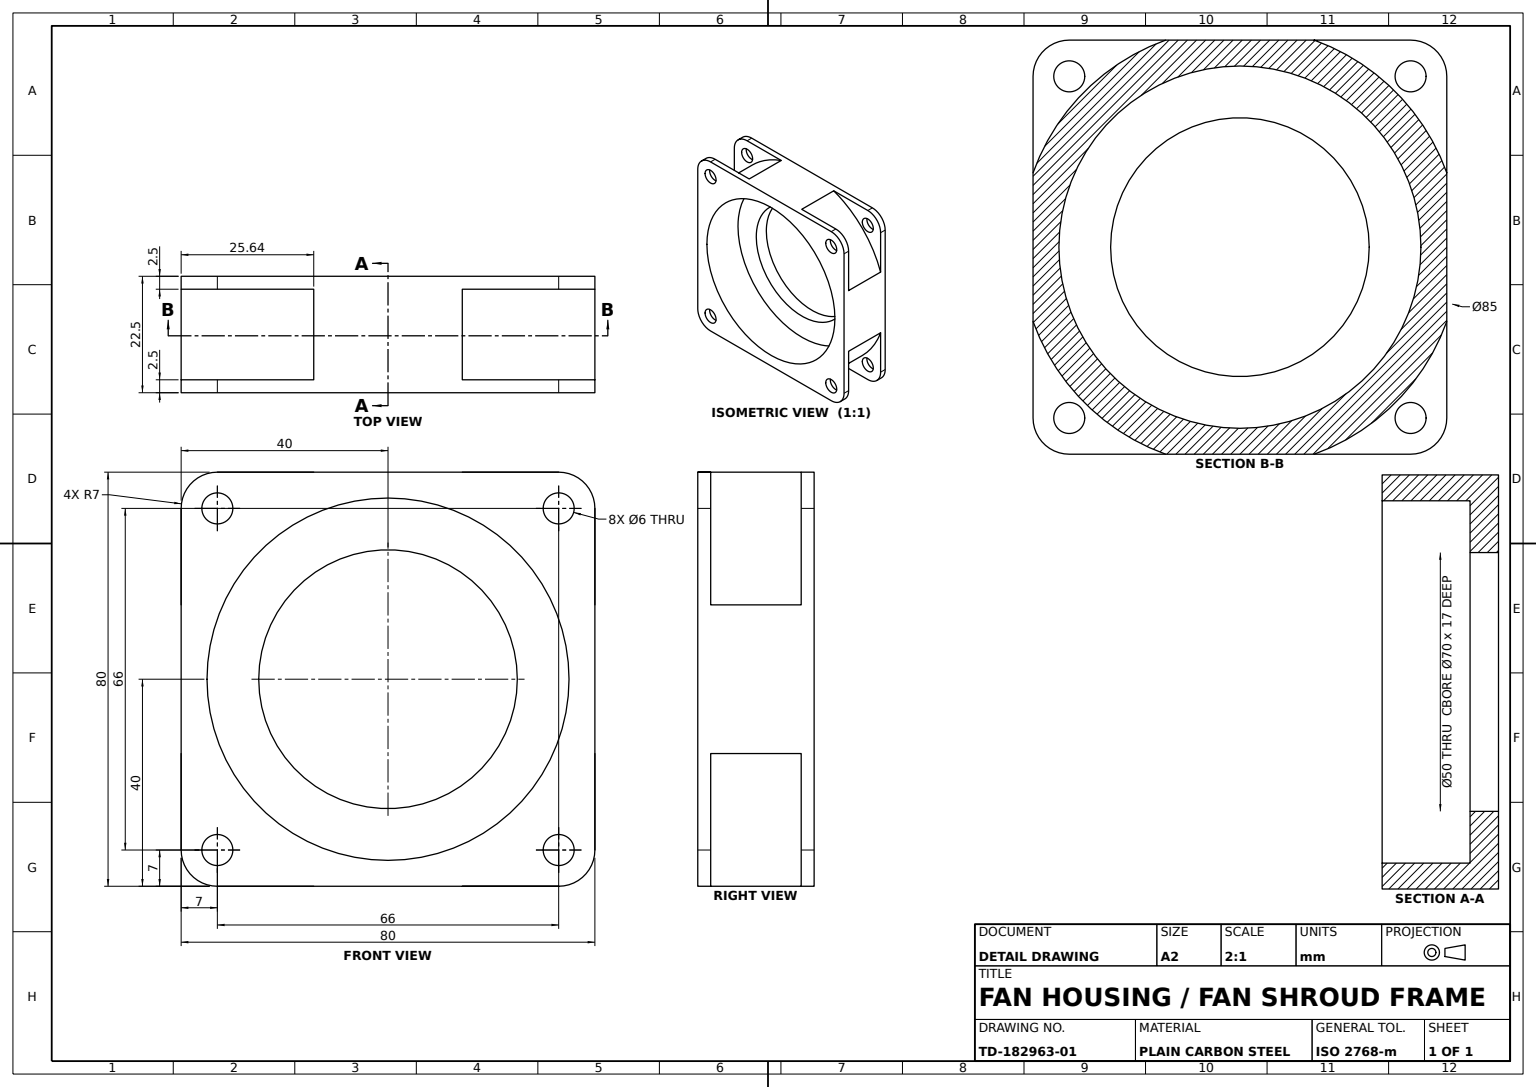
SolidWorks part; units mm, degrees
material "Plain Carbon Steel"
ref_plane "Front Plane" through (0, 0, 0) normal (0, 0, 1) x (1, 0, 0)
ref_plane "Top Plane" through (0, 0, 0) normal (0, 1, 0) x (1, 0, 0)
ref_plane "Right Plane" through (0, 0, 0) normal (1, 0, 0) x (0, 0, -1)
sketch "Front Flange Sketch" plane through (0, 0, 0) normal (0, 0, 1) x (1, 0, 0)
  line L0 (0, 0) -> (33, 0)
  line L1 (40, 7) -> (40, 73)
  line L2 (33, 80) -> (-33, 80)
  line L3 (-40, 73) -> (-40, 7)
  line L4 (-33, 0) -> (0, 0)
  arc A0 (33, 0) -> (40, 7) centre (33, 7) ccw
  arc A1 (-33, 0) -> (-40, 7) centre (-33, 7) cw
  arc A2 (40, 73) -> (33, 80) centre (33, 73) ccw
  arc A3 (-40, 73) -> (-33, 80) centre (-33, 73) cw
  point P8 (40, 0)
  point P11 (-40, 0)
  point P14 (40, 80)
  point P17 (-40, 80)
  dimension "D5" = 7
  dimension "D1" = 40
  dimension "D2" = 80
  dimension "D3" = 80
  dimension "D4" = 80
extrude "Front Flange 80x80" add sketch "Front Flange Sketch" along normal blind 2.5
sketch "Hub Sketch" plane through (0, 0, 2.5) normal (0, 0, 1) x (1, 0, 0)
  line L0 (40, 7) -> (40, 73) construction
  line L1 (-33, 0) -> (33, 0) construction
  circle A0 centre (0, 40) radius 35
  dimension "D1" = 70
  dimension "D2" = 40
  dimension "D3" = 40
extrude "Hub Ø70" add sketch "Hub Sketch" along normal blind 20
sketch "Rear Flange Sketch" plane through (0, 0, 22.5) normal (0, 0, 1) x (1, 0, 0)
  line L0 (0, 40) -> (40, 40)
  line L1 (40, 7) -> (40, 73) construction
  line L2 (40, 40) -> (40, 73)
  line L3 (33, 80) -> (-33, 80)
  line L4 (-40, 73) -> (-40, 7)
  line L5 (-33, 0) -> (33, 0)
  line L6 (40, 7) -> (40, 40)
  arc A0 (-33, 0) -> (-40, 7) centre (-33, 7) cw
  arc A1 (33, 0) -> (40, 7) centre (33, 7) ccw
  arc A2 (40, 73) -> (33, 80) centre (33, 73) ccw
  arc A3 (-33, 80) -> (-40, 73) centre (-33, 73) ccw
  point P12 (-40, 0)
  point P15 (40, 0)
  point P18 (40, 80)
  point P21 (-40, 80)
  dimension "D5" = 7
  dimension "D1" = 40
  dimension "D2" = 80
  dimension "D3" = 80
  dimension "D4" = 80
extrude "Rear Flange 80x80" add sketch "Rear Flange Sketch" against normal blind 2.5
sketch "Side Web Sketch" plane through (0, 0, 22.5) normal (0, 0, 1) x (1, 0, 0)
  line L0 (-14.3614, 80) -> (14.3614, 80)
  line L1 (-40, 54.3614) -> (-40, 25.6386)
  line L2 (-14.3614, 0) -> (14.3614, 0)
  line L4 (40, 54.3614) -> (40, 25.6386)
  arc A0 (-14.3614, 80) -> (-40, 54.3614) centre (0, 40) ccw
  arc A2 (-40, 25.6386) -> (-14.3614, 0) centre (0, 40) ccw
  arc A3 (14.3614, 0) -> (40, 25.6386) centre (0, 40) ccw
  arc A4 (40, 54.3614) -> (14.3614, 80) centre (0, 40) ccw
  dimension "D1" = 85
  dimension "D5" = 25.6386
  dimension "D2" = 40
  dimension "D3" = 80
  dimension "D4" = 40
  dimension "D6" = 25.6386
extrude "Side Webs" add sketch "Side Web Sketch" against normal blind 20
sketch "Large Bore Sketch" plane through (0, 0, 22.5) normal (0, 0, 1) x (1, 0, 0)
  line L0 (40, 7) -> (40, 73) construction
  line L1 (33, 80) -> (-33, 80) construction
  circle A0 centre (0, 40) radius 35
  dimension "D1" = 70
  dimension "D2" = 40
  dimension "D3" = 40
extrude "Large Bore Ø70" cut sketch "Large Bore Sketch" against normal blind 17
sketch "Through Bore Sketch" plane through (0, 0, 5.5) normal (0, 0, 1) x (1, 0, 0)
  circle A0 centre (0, 40) radius 25
  dimension "D1" = 50
extrude "Through Bore Ø50" cut sketch "Through Bore Sketch" against normal blind 8
sketch "Corner Holes Sketch" plane through (0, 0, 22.5) normal (0, 0, 1) x (1, 0, 0)
  circle A0 centre (-33, 73) radius 3
  circle A1 centre (33, 73) radius 3
  circle A2 centre (-33, 7) radius 3
  circle A3 centre (33, 7) radius 3
  dimension "D1" = 6
  dimension "D2" = 6
  dimension "D3" = 6
  dimension "D4" = 6
extrude "Corner Holes 4xØ6" cut sketch "Corner Holes Sketch" against normal blind 25
